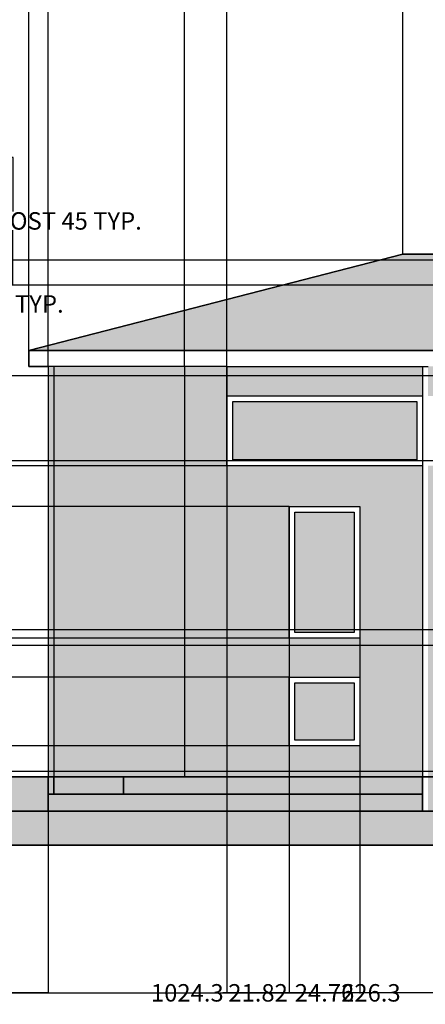
# Model space of a CAD drawing. Units: inches. Extents: x -655 to 499, y 20 to 616.
# Tile 4 of 7: x -137 to 5, y 20 to 365. Entities that reach past the tile are written whole.
import ezdxf

# ---------------------------------------------------------------- set-up
doc = ezdxf.new("R2010")
doc.units = ezdxf.units.IN
doc.header["$MEASUREMENT"] = 0
for name, color, linetype, lineweight in [('A-ANNO-DIMS', 2, 'Continuous', 18), ('A-DOOR', 4, 'Continuous', 25), ('A-ELEV', 7, 'Continuous', 35), ('A-ELEV-PATT', 9, 'Continuous', 13), ('A-ROOF', 1, 'Continuous', 35), ('C-TOPO', 18, 'Continuous', 18)]:
    doc.layers.add(name, color=color, linetype=linetype, lineweight=lineweight)
doc.styles.get("Standard").update_dxf_attribs({"font": 'arial.ttf'})
doc.dimstyles.get("Standard").update_dxf_attribs({"dimtxt": 6.125, "dimasz": 0.18, "dimexe": 0.18, "dimexo": 0.0625, "dimgap": 0.09, "dimtad": 0, "dimtih": 1, "dimtoh": 1, "dimdec": 4, "dimzin": 0, "dimdsep": 46, "dimlunit": 4, "dimtxsty": 'Standard', "dimcen": 0.09, "dimadec": 0, "dimazin": 0, "dimtfac": 1, "dimtdec": 4, "dimtofl": 0, "dimtmove": 0, "dimatfit": 3, "dimfxl": 1, "dimtolj": 1, "dimtzin": 0, "dimarcsym": 0})

# ---------------------------------------------------------------- blocks, each defined once
blk = doc.blocks.new('DOOR-LEAF-PANEL')
for points in [[(0, 122.75), (68.54, 122.75), (68.54, 98.27), (0, 98.27)], [(2, 120.75), (66.54, 120.75), (66.54, 100.27), (2, 100.27)], [(21.82, 83.95), (46.58, 83.95), (46.58, 37.78), (21.82, 37.78)], [(23.82, 81.95), (44.58, 81.95), (44.58, 39.78), (23.82, 39.78)], [(21.82, 24.14), (46.58, 24.14), (46.58, 0), (21.82, 0)], [(23.82, 22.14), (44.58, 22.14), (44.58, 2), (23.82, 2)]]:
    blk.add_lwpolyline(points, close=True)
blk = doc.blocks.new('*D4')
at = {"layer": 'A-ANNO-DIMS', "color": 0, "lineweight": -2, "transparency": 16777216}
for p, q in [((-145.9, 317.05), (-139.06, 317.05)), ((-139.24, 316.87), (-139.24, 297.92)), ((-139.24, 272.44), (-139.24, 291.4)), ((-145.9, 272.26), (-139.06, 272.26))]:
    blk.add_line(p, q, dxfattribs=at)
at = {"layer": 'A-ANNO-DIMS', "color": 0, "transparency": 16777216}
for points in [[(-139.27, 316.87), (-139.21, 316.87), (-139.24, 317.05)], [(-139.27, 272.44), (-139.21, 272.44), (-139.24, 272.26)]]:
    blk.add_solid(points, dxfattribs=at)
at = {"layer": 'Defpoints', "color": 0, "transparency": 16777216}
for p in [(-145.96, 317.05), (-139.24, 317.05), (-145.96, 272.26)]:
    blk.add_point(p, dxfattribs=at)
at = {"layer": 'A-ANNO-DIMS', "color": 0, "transparency": 16777216, "insert": (-139.24, 294.66), "char_height": 6.125, "attachment_point": 5}
blk.add_mtext('\\A1;BALCONY POST 45 TYP.', dxfattribs=at)
blk = doc.blocks.new('*D5')
at = {"layer": 'A-ANNO-DIMS', "color": 0, "lineweight": -2, "transparency": 16777216}
for p, q in [((-150.77, 272.2), (-150.77, 265.36)), ((-145.96, 272.2), (-145.96, 265.36)), ((-150.59, 265.54), (-146.14, 265.54)), ((-145.96, 265.54), (-145.78, 265.54))]:
    blk.add_line(p, q, dxfattribs=at)
at = {"layer": 'A-ANNO-DIMS', "color": 0, "transparency": 16777216}
for points in [[(-150.59, 265.57), (-150.59, 265.51), (-150.77, 265.54)], [(-146.14, 265.57), (-146.14, 265.51), (-145.96, 265.54)]]:
    blk.add_solid(points, dxfattribs=at)
at = {"layer": 'Defpoints', "color": 0, "transparency": 16777216}
for p in [(-150.77, 272.26), (-145.96, 272.26), (-145.96, 265.54)]:
    blk.add_point(p, dxfattribs=at)
at = {"layer": 'A-ANNO-DIMS', "color": 0, "transparency": 16777216, "insert": (-133.16, 265.54), "char_height": 6.125, "attachment_point": 5}
blk.add_mtext('\\A1;5 TYP.', dxfattribs=at)
blk = doc.blocks.new('*D10')
at = {"layer": 'A-ANNO-DIMS', "color": 0, "lineweight": -2, "transparency": 16777216}
for p, q in [((434.11, 393.11), (434.11, 23.7)), ((-590.16, 75.57), (-590.16, 23.7)), ((-589.98, 23.88), (-90.54, 23.88)), ((433.93, 23.88), (-65.51, 23.88))]:
    blk.add_line(p, q, dxfattribs=at)
at = {"layer": 'A-ANNO-DIMS', "color": 0, "transparency": 16777216}
for points in [[(-589.98, 23.91), (-589.98, 23.85), (-590.16, 23.88)], [(433.93, 23.91), (433.93, 23.85), (434.11, 23.88)]]:
    blk.add_solid(points, dxfattribs=at)
at = {"layer": 'Defpoints', "color": 0, "transparency": 16777216}
for p in [(434.11, 393.17), (-590.16, 75.63), (434.11, 23.88)]:
    blk.add_point(p, dxfattribs=at)
at = {"layer": 'A-ANNO-DIMS', "color": 0, "transparency": 16777216, "insert": (-78.02, 23.88), "char_height": 6.125, "attachment_point": 5}
blk.add_mtext('\\A1;1024.3', dxfattribs=at)
blk = doc.blocks.new('*D14')
at = {"layer": 'A-ANNO-DIMS', "color": 0, "lineweight": -2, "transparency": 16777216}
for p, q in [((-229.01, 101.57), (-229.01, 23.7)), ((-126.81, 99.57), (-126.81, 23.7)), ((-228.83, 23.88), (-188.01, 23.88)), ((-126.99, 23.88), (-167.8, 23.88))]:
    blk.add_line(p, q, dxfattribs=at)
at = {"layer": 'A-ANNO-DIMS', "color": 0, "transparency": 16777216}
for points in [[(-228.83, 23.91), (-228.83, 23.85), (-229.01, 23.88)], [(-126.99, 23.91), (-126.99, 23.85), (-126.81, 23.88)]]:
    blk.add_solid(points, dxfattribs=at)
at = {"layer": 'Defpoints', "color": 0, "transparency": 16777216}
for p in [(-229.01, 101.63), (-126.81, 99.63), (-126.81, 23.88)]:
    blk.add_point(p, dxfattribs=at)
at = {"layer": 'A-ANNO-DIMS', "color": 0, "transparency": 16777216, "insert": (-177.91, 23.88), "char_height": 6.125, "attachment_point": 5}
blk.add_mtext('\\A1;102.2', dxfattribs=at)
blk = doc.blocks.new('*D15')
at = {"layer": 'A-ANNO-DIMS', "color": 0, "lineweight": -2, "transparency": 16777216}
for p, q in [((-126.81, 99.57), (-126.81, 23.7)), ((99.5, 93.57), (99.5, 23.7)), ((-126.63, 23.88), (-24.13, 23.88)), ((99.32, 23.88), (-3.18, 23.88))]:
    blk.add_line(p, q, dxfattribs=at)
at = {"layer": 'A-ANNO-DIMS', "color": 0, "transparency": 16777216}
for points in [[(-126.63, 23.91), (-126.63, 23.85), (-126.81, 23.88)], [(99.32, 23.91), (99.32, 23.85), (99.5, 23.88)]]:
    blk.add_solid(points, dxfattribs=at)
at = {"layer": 'Defpoints', "color": 0, "transparency": 16777216}
for p in [(-126.81, 99.63), (99.5, 93.63), (99.5, 23.88)]:
    blk.add_point(p, dxfattribs=at)
at = {"layer": 'A-ANNO-DIMS', "color": 0, "transparency": 16777216, "insert": (-13.65, 23.88), "char_height": 6.125, "attachment_point": 5}
blk.add_mtext('\\A1;226.3', dxfattribs=at)
blk = doc.blocks.new('*D21')
at = {"layer": 'A-ANNO-DIMS', "color": 0, "lineweight": -2, "transparency": 16777216}
for p, q in [((179.11, 559.78), (486.04, 559.78)), ((485.86, 559.6), (485.86, 320.92)), ((485.86, 75.81), (485.86, 314.49)), ((-590.1, 75.63), (486.04, 75.63))]:
    blk.add_line(p, q, dxfattribs=at)
at = {"layer": 'A-ANNO-DIMS', "color": 0, "transparency": 16777216}
for points in [[(485.83, 559.6), (485.89, 559.6), (485.86, 559.78)], [(485.83, 75.81), (485.89, 75.81), (485.86, 75.63)]]:
    blk.add_solid(points, dxfattribs=at)
at = {"layer": 'Defpoints', "color": 0, "transparency": 16777216}
for p in [(179.05, 559.78), (485.86, 559.78), (-590.16, 75.63)]:
    blk.add_point(p, dxfattribs=at)
at = {"layer": 'A-ANNO-DIMS', "color": 0, "transparency": 16777216, "insert": (485.86, 317.7), "char_height": 6.125, "attachment_point": 5}
blk.add_mtext('\\A1;484.15', dxfattribs=at)
blk = doc.blocks.new('*D35')
at = {"layer": 'A-ANNO-DIMS', "color": 0, "lineweight": -2, "transparency": 16777216}
for p, q in [((-244.62, 280.97), (486.04, 280.97)), ((485.86, 280.79), (485.86, 279.83)), ((485.86, 272.44), (485.86, 273.4)), ((-226.95, 272.26), (486.04, 272.26))]:
    blk.add_line(p, q, dxfattribs=at)
at = {"layer": 'A-ANNO-DIMS', "color": 0, "transparency": 16777216}
for points in [[(485.83, 280.79), (485.89, 280.79), (485.86, 280.97)], [(485.83, 272.44), (485.89, 272.44), (485.86, 272.26)]]:
    blk.add_solid(points, dxfattribs=at)
at = {"layer": 'Defpoints', "color": 0, "transparency": 16777216}
for p in [(-244.69, 280.97), (-227.01, 272.26), (485.86, 272.26)]:
    blk.add_point(p, dxfattribs=at)
at = {"layer": 'A-ANNO-DIMS', "color": 0, "transparency": 16777216, "insert": (485.86, 276.61), "char_height": 6.125, "attachment_point": 5}
blk.add_mtext('\\A1;8.706', dxfattribs=at)
blk = doc.blocks.new('*D48')
at = {"layer": 'A-ANNO-DIMS', "color": 0, "lineweight": -2, "transparency": 16777216}
for p, q in [((-228.95, 145.8), (486.04, 145.8)), ((485.86, 145.62), (485.86, 126.88)), ((485.86, 101.81), (485.86, 120.55)), ((-228.95, 101.63), (486.04, 101.63))]:
    blk.add_line(p, q, dxfattribs=at)
at = {"layer": 'A-ANNO-DIMS', "color": 0, "transparency": 16777216}
for points in [[(485.83, 145.62), (485.89, 145.62), (485.86, 145.8)], [(485.83, 101.81), (485.89, 101.81), (485.86, 101.63)]]:
    blk.add_solid(points, dxfattribs=at)
at = {"layer": 'Defpoints', "color": 0, "transparency": 16777216}
for p in [(-229.01, 145.8), (485.86, 145.8), (-229.01, 101.63)]:
    blk.add_point(p, dxfattribs=at)
at = {"layer": 'A-ANNO-DIMS', "color": 0, "transparency": 16777216, "insert": (485.86, 123.72), "char_height": 6.125, "attachment_point": 5}
blk.add_mtext('\\A1;44.17', dxfattribs=at)
blk = doc.blocks.new('*D49')
at = {"layer": 'A-ANNO-DIMS', "color": 0, "lineweight": -2, "transparency": 16777216}
for p, q in [((-229.3, 210.64), (486.04, 210.64)), ((485.86, 210.46), (485.86, 184.21)), ((485.86, 151.52), (485.86, 177.77)), ((-229.3, 151.34), (486.04, 151.34))]:
    blk.add_line(p, q, dxfattribs=at)
at = {"layer": 'A-ANNO-DIMS', "color": 0, "transparency": 16777216}
for points in [[(485.83, 210.46), (485.89, 210.46), (485.86, 210.64)], [(485.83, 151.52), (485.89, 151.52), (485.86, 151.34)]]:
    blk.add_solid(points, dxfattribs=at)
at = {"layer": 'Defpoints', "color": 0, "transparency": 16777216}
for p in [(-229.36, 210.64), (485.86, 210.64), (-229.36, 151.34)]:
    blk.add_point(p, dxfattribs=at)
at = {"layer": 'A-ANNO-DIMS', "color": 0, "transparency": 16777216, "insert": (485.86, 180.99), "char_height": 6.125, "attachment_point": 5}
blk.add_mtext('\\A1;59.3', dxfattribs=at)
blk = doc.blocks.new('*D51')
at = {"layer": 'A-ANNO-DIMS', "color": 0, "lineweight": -2, "transparency": 16777216}
for p, q in [((-228.95, 240.42), (486.04, 240.42)), ((485.86, 240.24), (485.86, 228.75)), ((485.86, 210.82), (485.86, 222.31)), ((-228.88, 210.64), (486.04, 210.64))]:
    blk.add_line(p, q, dxfattribs=at)
at = {"layer": 'A-ANNO-DIMS', "color": 0, "transparency": 16777216}
for points in [[(485.83, 240.24), (485.89, 240.24), (485.86, 240.42)], [(485.83, 210.82), (485.89, 210.82), (485.86, 210.64)]]:
    blk.add_solid(points, dxfattribs=at)
at = {"layer": 'Defpoints', "color": 0, "transparency": 16777216}
for p in [(-229.01, 240.42), (485.86, 240.42), (-228.94, 210.64)]:
    blk.add_point(p, dxfattribs=at)
at = {"layer": 'A-ANNO-DIMS', "color": 0, "transparency": 16777216, "insert": (485.86, 225.53), "char_height": 6.125, "attachment_point": 5}
blk.add_mtext('\\A1;29.776', dxfattribs=at)
blk = doc.blocks.new('*D55')
at = {"layer": 'A-ANNO-DIMS', "color": 0, "lineweight": -2, "transparency": 16777216}
for p, q in [((-133.53, 249.26), (-133.53, 611.71)), ((-133.35, 611.53), (-80.53, 611.53)), ((-2.68, 611.53), (-55.5, 611.53)), ((-2.5, 283.02), (-2.5, 611.71))]:
    blk.add_line(p, q, dxfattribs=at)
at = {"layer": 'A-ANNO-DIMS', "color": 0, "transparency": 16777216}
for points in [[(-133.35, 611.56), (-133.35, 611.5), (-133.53, 611.53)], [(-2.68, 611.56), (-2.68, 611.5), (-2.5, 611.53)]]:
    blk.add_solid(points, dxfattribs=at)
at = {"layer": 'Defpoints', "color": 0, "transparency": 16777216}
for p in [(-2.5, 611.53), (-2.5, 282.96), (-133.53, 249.2)]:
    blk.add_point(p, dxfattribs=at)
at = {"layer": 'A-ANNO-DIMS', "color": 0, "transparency": 16777216, "insert": (-68.01, 611.53), "char_height": 6.125, "attachment_point": 5}
blk.add_mtext('\\A1;131.03', dxfattribs=at)
blk = doc.blocks.new('*D56')
at = {"layer": 'A-ANNO-DIMS', "color": 0, "lineweight": -2, "transparency": 16777216}
for p, q in [((-2.5, 283.02), (-2.5, 611.71)), ((-2.32, 611.53), (46.26, 611.53)), ((115.13, 611.53), (66.55, 611.53)), ((115.31, 249.31), (115.31, 611.71))]:
    blk.add_line(p, q, dxfattribs=at)
at = {"layer": 'A-ANNO-DIMS', "color": 0, "transparency": 16777216}
for points in [[(-2.32, 611.56), (-2.32, 611.5), (-2.5, 611.53)], [(115.13, 611.56), (115.13, 611.5), (115.31, 611.53)]]:
    blk.add_solid(points, dxfattribs=at)
at = {"layer": 'Defpoints', "color": 0, "transparency": 16777216}
for p in [(115.31, 611.53), (-2.5, 282.96), (115.31, 249.25)]:
    blk.add_point(p, dxfattribs=at)
at = {"layer": 'A-ANNO-DIMS', "color": 0, "transparency": 16777216, "insert": (56.41, 611.53), "char_height": 6.125, "attachment_point": 5}
blk.add_mtext('\\A1;117.8', dxfattribs=at)
blk = doc.blocks.new('*D59')
at = {"layer": 'A-ANNO-DIMS', "color": 0, "lineweight": -2, "transparency": 16777216}
for p, q in [((-126.81, 243.69), (-126.81, 611.71)), ((-126.63, 611.53), (-113.42, 611.53)), ((-79.15, 611.53), (-92.35, 611.53)), ((-78.97, 243.69), (-78.97, 611.71))]:
    blk.add_line(p, q, dxfattribs=at)
at = {"layer": 'A-ANNO-DIMS', "color": 0, "transparency": 16777216}
for points in [[(-126.63, 611.56), (-126.63, 611.5), (-126.81, 611.53)], [(-79.15, 611.56), (-79.15, 611.5), (-78.97, 611.53)]]:
    blk.add_solid(points, dxfattribs=at)
at = {"layer": 'Defpoints', "color": 0, "transparency": 16777216}
for p in [(-78.97, 611.53), (-126.81, 243.63), (-78.97, 243.63)]:
    blk.add_point(p, dxfattribs=at)
at = {"layer": 'A-ANNO-DIMS', "color": 0, "transparency": 16777216, "insert": (-102.89, 611.53), "char_height": 6.125, "attachment_point": 5}
blk.add_mtext('\\A1;47.84', dxfattribs=at)
blk = doc.blocks.new('*D60')
at = {"layer": 'A-ANNO-DIMS', "color": 0, "lineweight": -2, "transparency": 16777216}
for p, q in [((-78.97, 243.69), (-78.97, 611.71)), ((-78.79, 611.53), (-64.3, 611.53)), ((-64.12, 233.34), (-64.12, 611.71)), ((-64.12, 611.53), (-63.94, 611.53))]:
    blk.add_line(p, q, dxfattribs=at)
at = {"layer": 'A-ANNO-DIMS', "color": 0, "transparency": 16777216}
for points in [[(-78.79, 611.56), (-78.79, 611.5), (-78.97, 611.53)], [(-64.3, 611.56), (-64.3, 611.5), (-64.12, 611.53)]]:
    blk.add_solid(points, dxfattribs=at)
at = {"layer": 'Defpoints', "color": 0, "transparency": 16777216}
for p in [(-64.12, 611.53), (-78.97, 243.63), (-64.12, 233.27)]:
    blk.add_point(p, dxfattribs=at)
at = {"layer": 'A-ANNO-DIMS', "color": 0, "transparency": 16777216, "insert": (-53.78, 611.53), "char_height": 6.125, "attachment_point": 5}
blk.add_mtext('\\A1;14.85', dxfattribs=at)
blk = doc.blocks.new('*D61')
at = {"layer": 'A-ANNO-DIMS', "color": 0, "lineweight": -2, "transparency": 16777216}
for p, q in [((-64.12, 233.34), (-64.12, 611.71)), ((-63.94, 611.53), (0.16, 611.53)), ((89.22, 611.53), (25.13, 611.53)), ((89.4, 243.69), (89.4, 611.71))]:
    blk.add_line(p, q, dxfattribs=at)
at = {"layer": 'A-ANNO-DIMS', "color": 0, "transparency": 16777216}
for points in [[(-63.94, 611.56), (-63.94, 611.5), (-64.12, 611.53)], [(89.22, 611.56), (89.22, 611.5), (89.4, 611.53)]]:
    blk.add_solid(points, dxfattribs=at)
at = {"layer": 'Defpoints', "color": 0, "transparency": 16777216}
for p in [(89.4, 611.53), (89.4, 243.63), (-64.12, 233.27)]:
    blk.add_point(p, dxfattribs=at)
at = {"layer": 'A-ANNO-DIMS', "color": 0, "transparency": 16777216, "insert": (12.64, 611.53), "char_height": 6.125, "attachment_point": 5}
blk.add_mtext('\\A1;153.52', dxfattribs=at)
blk = doc.blocks.new('*D65')
at = {"layer": 'A-ANNO-DIMS', "color": 0, "lineweight": -2, "transparency": 16777216}
for p, q in [((-64.12, 208.73), (-64.12, 23.7)), ((-42.3, 194.41), (-42.3, 23.7)), ((-63.94, 23.88), (-63.65, 23.88)), ((-42.48, 23.88), (-42.76, 23.88))]:
    blk.add_line(p, q, dxfattribs=at)
at = {"layer": 'A-ANNO-DIMS', "color": 0, "transparency": 16777216}
for points in [[(-63.94, 23.91), (-63.94, 23.85), (-64.12, 23.88)], [(-42.48, 23.91), (-42.48, 23.85), (-42.3, 23.88)]]:
    blk.add_solid(points, dxfattribs=at)
at = {"layer": 'Defpoints', "color": 0, "transparency": 16777216}
for p in [(-64.12, 208.79), (-42.3, 194.47), (-42.3, 23.88)]:
    blk.add_point(p, dxfattribs=at)
at = {"layer": 'A-ANNO-DIMS', "color": 0, "transparency": 16777216, "insert": (-53.21, 23.88), "char_height": 6.125, "attachment_point": 5}
blk.add_mtext('\\A1;21.82', dxfattribs=at)
blk = doc.blocks.new('*D66')
at = {"layer": 'A-ANNO-DIMS', "color": 0, "lineweight": -2, "transparency": 16777216}
for p, q in [((-42.3, 194.41), (-42.3, 23.7)), ((-17.54, 194.41), (-17.54, 23.7)), ((-42.12, 23.88), (-40.39, 23.88)), ((-17.72, 23.88), (-19.44, 23.88))]:
    blk.add_line(p, q, dxfattribs=at)
at = {"layer": 'A-ANNO-DIMS', "color": 0, "transparency": 16777216}
for points in [[(-42.12, 23.91), (-42.12, 23.85), (-42.3, 23.88)], [(-17.72, 23.91), (-17.72, 23.85), (-17.54, 23.88)]]:
    blk.add_solid(points, dxfattribs=at)
at = {"layer": 'Defpoints', "color": 0, "transparency": 16777216}
for p in [(-42.3, 194.47), (-17.54, 194.47), (-17.54, 23.88)]:
    blk.add_point(p, dxfattribs=at)
at = {"layer": 'A-ANNO-DIMS', "color": 0, "transparency": 16777216, "insert": (-29.92, 23.88), "char_height": 6.125, "attachment_point": 5}
blk.add_mtext('\\A1;24.76', dxfattribs=at)
blk = doc.blocks.new('*D67')
at = {"layer": 'A-ANNO-DIMS', "color": 0, "lineweight": -2, "transparency": 16777216}
for p, q in [((-42.36, 110.53), (-642.09, 110.53)), ((-641.91, 110.35), (-641.91, 108.29)), ((-641.91, 99.81), (-641.91, 101.86)), ((-64.18, 99.63), (-642.09, 99.63))]:
    blk.add_line(p, q, dxfattribs=at)
at = {"layer": 'A-ANNO-DIMS', "color": 0, "transparency": 16777216}
for points in [[(-641.94, 110.35), (-641.88, 110.35), (-641.91, 110.53)], [(-641.94, 99.81), (-641.88, 99.81), (-641.91, 99.63)]]:
    blk.add_solid(points, dxfattribs=at)
at = {"layer": 'Defpoints', "color": 0, "transparency": 16777216}
for p in [(-42.3, 110.53), (-641.91, 99.63), (-64.12, 99.63)]:
    blk.add_point(p, dxfattribs=at)
at = {"layer": 'A-ANNO-DIMS', "color": 0, "transparency": 16777216, "insert": (-641.91, 105.08), "char_height": 6.125, "attachment_point": 5}
blk.add_mtext('\\A1;10.896', dxfattribs=at)
blk = doc.blocks.new('*D68')
at = {"layer": 'A-ANNO-DIMS', "color": 0, "lineweight": -2, "transparency": 16777216}
for p, q in [((-42.36, 134.67), (-642.09, 134.67)), ((-641.91, 134.49), (-641.91, 125.76)), ((-641.91, 110.71), (-641.91, 119.43)), ((-42.36, 110.53), (-642.09, 110.53))]:
    blk.add_line(p, q, dxfattribs=at)
at = {"layer": 'A-ANNO-DIMS', "color": 0, "transparency": 16777216}
for points in [[(-641.94, 134.49), (-641.88, 134.49), (-641.91, 134.67)], [(-641.94, 110.71), (-641.88, 110.71), (-641.91, 110.53)]]:
    blk.add_solid(points, dxfattribs=at)
at = {"layer": 'Defpoints', "color": 0, "transparency": 16777216}
for p in [(-641.91, 134.67), (-42.3, 134.67), (-42.3, 110.53)]:
    blk.add_point(p, dxfattribs=at)
at = {"layer": 'A-ANNO-DIMS', "color": 0, "transparency": 16777216, "insert": (-641.91, 122.6), "char_height": 6.125, "attachment_point": 5}
blk.add_mtext('\\A1;24.14', dxfattribs=at)
blk = doc.blocks.new('*D69')
at = {"layer": 'A-ANNO-DIMS', "color": 0, "lineweight": -2, "transparency": 16777216}
for p, q in [((-42.36, 148.31), (-642.09, 148.31)), ((-641.91, 148.13), (-641.91, 144.71)), ((-641.91, 134.85), (-641.91, 138.27)), ((-42.36, 134.67), (-642.09, 134.67))]:
    blk.add_line(p, q, dxfattribs=at)
at = {"layer": 'A-ANNO-DIMS', "color": 0, "transparency": 16777216}
for points in [[(-641.94, 148.13), (-641.88, 148.13), (-641.91, 148.31)], [(-641.94, 134.85), (-641.88, 134.85), (-641.91, 134.67)]]:
    blk.add_solid(points, dxfattribs=at)
at = {"layer": 'Defpoints', "color": 0, "transparency": 16777216}
for p in [(-641.91, 148.31), (-42.3, 148.31), (-42.3, 134.67)]:
    blk.add_point(p, dxfattribs=at)
at = {"layer": 'A-ANNO-DIMS', "color": 0, "transparency": 16777216, "insert": (-641.91, 141.49), "char_height": 6.125, "attachment_point": 5}
blk.add_mtext('\\A1;13.64', dxfattribs=at)
blk = doc.blocks.new('*D70')
at = {"layer": 'A-ANNO-DIMS', "color": 0, "lineweight": -2, "transparency": 16777216}
for p, q in [((-42.36, 194.47), (-642.09, 194.47)), ((-641.91, 194.29), (-641.91, 174.61)), ((-641.91, 148.49), (-641.91, 168.17)), ((-42.36, 148.31), (-642.09, 148.31))]:
    blk.add_line(p, q, dxfattribs=at)
at = {"layer": 'A-ANNO-DIMS', "color": 0, "transparency": 16777216}
for points in [[(-641.94, 194.29), (-641.88, 194.29), (-641.91, 194.47)], [(-641.94, 148.49), (-641.88, 148.49), (-641.91, 148.31)]]:
    blk.add_solid(points, dxfattribs=at)
at = {"layer": 'Defpoints', "color": 0, "transparency": 16777216}
for p in [(-641.91, 194.47), (-42.3, 194.47), (-42.3, 148.31)]:
    blk.add_point(p, dxfattribs=at)
at = {"layer": 'A-ANNO-DIMS', "color": 0, "transparency": 16777216, "insert": (-641.91, 171.39), "char_height": 6.125, "attachment_point": 5}
blk.add_mtext('\\A1;46.16', dxfattribs=at)
blk = doc.blocks.new('*D71')
at = {"layer": 'A-ANNO-DIMS', "color": 0, "lineweight": -2, "transparency": 16777216}
for p, q in [((-64.18, 208.79), (-642.09, 208.79)), ((-641.91, 208.61), (-641.91, 204.85)), ((-641.91, 194.65), (-641.91, 198.41)), ((-42.36, 194.47), (-642.09, 194.47))]:
    blk.add_line(p, q, dxfattribs=at)
at = {"layer": 'A-ANNO-DIMS', "color": 0, "transparency": 16777216}
for points in [[(-641.94, 208.61), (-641.88, 208.61), (-641.91, 208.79)], [(-641.94, 194.65), (-641.88, 194.65), (-641.91, 194.47)]]:
    blk.add_solid(points, dxfattribs=at)
at = {"layer": 'Defpoints', "color": 0, "transparency": 16777216}
for p in [(-641.91, 208.79), (-64.12, 208.79), (-42.3, 194.47)]:
    blk.add_point(p, dxfattribs=at)
at = {"layer": 'A-ANNO-DIMS', "color": 0, "transparency": 16777216, "insert": (-641.91, 201.63), "char_height": 6.125, "attachment_point": 5}
blk.add_mtext('\\A1;14.32', dxfattribs=at)

msp = doc.modelspace()

# ---------------------------------------------------------------- hatches: boundary and pattern name
at = {"layer": 'A-ELEV-PATT'}
h = msp.add_hatch(color=256, dxfattribs=at)
h.dxf.hatch_style = 1
h.paths.add_polyline_path([(-140.0489, 272.2618), (-399.3758, 272.2618), (-399.3758, 249.8418), (-399.3758, 248.5179), (-366.9446, 248.7444), (-209.8047, 249.8418), (-183.5755, 249.8418), (-140.0489, 249.8418)])
h.paths.add_polyline_path([(-211.7589, 317.0515), (-216.5713, 317.0515), (-216.5713, 272.2618), (-211.7589, 272.2618)])
h.paths.add_polyline_path([(-145.96, 317.0515), (-150.7725, 317.0515), (-150.7725, 272.2618), (-145.96, 272.2618)])
h.paths.add_polyline_path([(-140.5198, 321.4867), (-402.0739, 321.4867), (-402.0739, 317.0515), (-390.1757, 317.0515), (-385.3633, 317.0515), (-150.7725, 317.0515), (-145.96, 317.0515), (-140.5198, 317.0515)])
h.paths.add_polyline_path([(-269.7123, 317.0515), (-274.5248, 317.0515), (-274.5248, 272.2618), (-269.7123, 272.2618)])
h.paths.add_polyline_path([(-329.7837, 317.0515), (-334.5961, 317.0515), (-334.5961, 280.9678), (-329.7837, 280.9678)])
h.paths.add_polyline_path([(-329.7837, 280.9678), (-334.5961, 280.9678), (-334.5961, 272.2618), (-329.7837, 272.2618)])
h.paths.add_polyline_path([(-385.3633, 317.0515), (-390.1757, 317.0515), (-390.1757, 272.2618), (-385.3633, 272.2618)])
h.paths.add_polyline_path([(-229.0087, 240.4184), (-354.3532, 240.4184), (-354.2854, 210.6425), (-315.9956, 210.6425), (-315.9956, 210.9348), (-277.6793, 210.7995), (-277.6793, 210.6425), (-273.1052, 210.6425), (-273.1052, 210.7995), (-229.3637, 210.6425), (-229.0087, 210.6425)])
h.paths.add_polyline_path([(-229.0087, 145.8007), (-354.3532, 145.8007), (-354.3532, 101.6296), (-229.0087, 101.6296)])
h.paths.add_polyline_path([(-229.0087, 210.6425), (-229.3637, 210.6425), (-229.3637, 151.3385), (-273.1052, 151.4955), (-273.1052, 210.6425), (-277.6793, 210.6425), (-277.6793, 151.4955), (-315.9956, 151.6308), (-315.9956, 210.6425), (-318.9742, 210.6425), (-318.9742, 151.3385), (-354.3532, 151.3385), (-354.3532, 145.8007), (-229.0087, 145.8007)])
h.paths.add_polyline_path([(-229.0087, 247.8418), (-354.3532, 247.8418), (-354.3532, 240.4184), (-229.0087, 240.4184)])
h.paths.add_polyline_path([(4.4271, 93.6296), (-100.4134, 93.6296), (-124.8077, 93.6296), (-126.8077, 93.6296), (-126.8077, 87.6296), (4.4271, 87.6296)])
h.paths.add_polyline_path([(4.4271, 99.6296), (-100.4134, 99.6296), (-100.4134, 93.6296), (4.4271, 93.6296)])
h.paths.add_polyline_path([(99.4982, 99.6296), (6.4271, 99.6296), (6.4271, 93.6296), (99.4982, 93.6296)])
h.paths.add_polyline_path([(99.4982, 93.6296), (6.4271, 93.6296), (6.4271, 87.6296), (99.4982, 87.6296)])
h.paths.add_polyline_path([(304.2843, 311.436), (230.0144, 311.076), (230.0144, 282.9577), (270.6361, 282.9577), (304.4665, 273.8535)])
h.paths.add_polyline_path([(304.1054, 348.3371), (304.1054, 356.2861), (230.0144, 356.2861), (230.0144, 348.3443), (230.0144, 311.076), (304.2843, 311.436)])
h.paths.add_polyline_path([(255.5586, 316.5111), (255.5586, 350.0185), (275.6848, 350.0185), (275.6848, 316.5111)], flags=16)
h.paths.add_polyline_path([(278.0676, 316.5111), (278.0676, 350.0185), (301.4074, 350.0185), (301.4074, 316.5111)], flags=16)
h.paths.add_polyline_path([(253.2029, 316.5111), (233.8107, 316.5111), (233.8107, 350.0185), (253.2029, 350.0185)], flags=16)
h.paths.add_polyline_path([(179.0482, 559.7795), (153.2347, 535.8185), (165.0976, 535.8185), (192.9989, 535.8185), (201.2897, 535.8185)])
h.paths.add_polyline_path([(347.8163, 516.7932), (322.0028, 492.8322), (333.8657, 492.8322), (361.7669, 492.8322), (370.0577, 492.8322)])
h = msp.add_hatch(color=256, dxfattribs=at)
h.dxf.hatch_style = 1
h.paths.add_polyline_path([(-329.7837, 350.1333), (-347.0336, 350.1333), (-347.0336, 321.4867), (-329.7837, 321.4867)])
h.paths.add_polyline_path([(-294.1413, 350.1333), (-311.3912, 350.1333), (-311.3912, 321.4867), (-294.1413, 321.4867)])
h.paths.add_polyline_path([(-294.1413, 317.0515), (-311.3912, 317.0515), (-311.3912, 280.9678), (-294.1413, 280.9678)])
h.paths.add_polyline_path([(-334.5961, 317.0515), (-347.0336, 317.0515), (-347.0336, 280.9678), (-334.5961, 280.9678)])
h.paths.add_polyline_path([(-244.6859, 336.719), (-258.4486, 336.719), (-258.4486, 347.0139), (-244.6859, 347.0139), (-244.6859, 350.1333), (-261.9358, 350.1333), (-261.9358, 321.4867), (-244.6859, 321.4867)])
h.paths.add_polyline_path([(-244.6859, 317.0515), (-261.9358, 317.0515), (-261.9358, 280.9678), (-244.6859, 280.9678)])
h.paths.add_polyline_path([(-244.6859, 347.0139), (-258.4486, 347.0139), (-258.4486, 336.719), (-244.6859, 336.719)], flags=17)
h.paths.add_polyline_path([(-318.9742, 210.6425), (-354.3532, 210.6425), (-354.3532, 151.3385), (-318.9742, 151.3385)])
h.paths.add_polyline_path([(-277.6793, 210.6425), (-315.9956, 210.6425), (-315.9956, 151.6308), (-277.6793, 151.4955)])
h.paths.add_polyline_path([(-229.3637, 210.6425), (-273.1052, 210.6425), (-273.1052, 151.4955), (-229.3637, 151.3385)])
h.paths.add_polyline_path([(-19.537, 192.4712), (-40.2951, 192.4712), (-40.2951, 150.3082), (-19.537, 150.3082)])
h.paths.add_polyline_path([(2.4271, 231.274), (-62.1158, 231.274), (-62.1158, 210.7923), (2.4271, 210.7923)])
h.paths.add_polyline_path([(72.97, 231.274), (8.4271, 231.274), (8.4271, 210.7923), (72.97, 210.7923)])
h.paths.add_polyline_path([(51.0059, 192.4712), (30.2478, 192.4712), (30.2478, 150.3082), (51.0059, 150.3082)])
h.paths.add_polyline_path([(51.0059, 132.6671), (30.2478, 132.6671), (30.2478, 112.5254), (51.0059, 112.5254)])
h.paths.add_polyline_path([(-19.537, 132.6671), (-40.2951, 132.6671), (-40.2951, 112.5254), (-19.537, 112.5254)])
h.paths.add_polyline_path([(275.6848, 350.0185), (255.5586, 350.0185), (255.5586, 316.5111), (275.6848, 316.5111)])
h.paths.add_polyline_path([(301.4074, 350.0185), (278.0676, 350.0185), (278.0676, 316.5111), (301.4074, 316.5111)])
h.paths.add_polyline_path([(253.2029, 350.0185), (233.8107, 350.0185), (233.8107, 316.5111), (253.2029, 316.5111)])
h = msp.add_hatch(color=256, dxfattribs=at)
h.dxf.hatch_style = 1
h.paths.add_polyline_path([(-126.8077, 93.6296), (-126.8077, 99.6296), (-145.6102, 99.6296), (-209.8047, 99.6296), (-366.9446, 98.5321), (-366.9446, 99.6296), (-506.835, 99.6296), (-573.6788, 99.6296), (-573.6788, 87.6296), (-506.835, 87.6296), (-161.7817, 87.6296), (-126.8077, 87.6296)])
h.paths.add_polyline_path([(419.8436, 99.6296), (99.4982, 99.6296), (99.4982, 87.6296), (419.8436, 87.6296)])
h.paths.add_polyline_path([(-100.4134, 99.6296), (-124.8077, 99.6296), (-124.8077, 93.6296), (-100.4134, 93.6296)])
h.paths.add_polyline_path([(-124.8077, 243.6296), (-126.8077, 243.6296), (-126.8077, 99.6296), (-124.8077, 99.6296)])
h.paths.add_polyline_path([(-124.8077, 99.6296), (-126.8077, 99.6296), (-126.8077, 93.6296), (-124.8077, 93.6296)])
h = msp.add_hatch(color=256, dxfattribs=at)
h.dxf.hatch_style = 1
h.paths.add_polyline_path([(-78.9669, 243.6296), (-124.8077, 243.6296), (-124.8077, 99.6296), (-78.9669, 99.6296)])
h.paths.add_polyline_path([(109.2763, 243.6296), (100.3937, 243.6296), (89.4008, 243.6296), (89.4008, 99.6296), (99.4982, 99.6296), (109.2763, 99.6296)])
h = msp.add_hatch(color=256, dxfattribs=at)
h.dxf.hatch_style = 1
h.paths.add_polyline_path([(-64.1158, 243.6296), (-78.9669, 243.6296), (-78.9669, 99.6296), (-64.1158, 99.6296)])
h.paths.add_polyline_path([(74.97, 243.6296), (18.4987, 243.6296), (6.4271, 243.6296), (6.4271, 233.274), (74.97, 233.274)])
h.paths.add_polyline_path([(4.4271, 243.6296), (4.3518, 243.6296), (4.0451, 243.6296), (-52.0442, 243.6296), (-64.1158, 243.6296), (-64.1158, 233.274), (4.4271, 233.274)])
h.paths.add_polyline_path([(89.4008, 243.6296), (74.97, 243.6296), (74.97, 233.274), (74.97, 99.6296), (89.4008, 99.6296)])
h.paths.add_polyline_path([(74.97, 208.7923), (6.4271, 208.7923), (6.4271, 99.6296), (74.97, 99.6296)])
h.paths.add_polyline_path([(53.0059, 148.3082), (28.2478, 148.3082), (28.2478, 194.4712), (53.0059, 194.4712)], flags=16)
h.paths.add_polyline_path([(51.0059, 150.3082), (30.2478, 150.3082), (30.2478, 192.4712), (51.0059, 192.4712)], flags=0)
h.paths.add_polyline_path([(53.0059, 134.6671), (53.0059, 110.5254), (28.2478, 110.5254), (28.2478, 134.6671)], flags=16)
h.paths.add_polyline_path([(51.0059, 132.6671), (51.0059, 112.5254), (30.2478, 112.5254), (30.2478, 132.6671)], flags=0)
h.paths.add_polyline_path([(4.4271, 208.7923), (-64.1158, 208.7923), (-64.1158, 99.6296), (4.4271, 99.6296)])
h.paths.add_polyline_path([(-17.537, 148.3082), (-42.2951, 148.3082), (-42.2951, 194.4712), (-17.537, 194.4712)], flags=16)
h.paths.add_polyline_path([(-19.537, 150.3082), (-40.2951, 150.3082), (-40.2951, 192.4712), (-19.537, 192.4712)], flags=0)
h.paths.add_polyline_path([(-17.537, 134.6671), (-17.537, 110.5254), (-42.2951, 110.5254), (-42.2951, 134.6671)], flags=16)
h.paths.add_polyline_path([(-19.537, 132.6671), (-19.537, 112.5254), (-40.2951, 112.5254), (-40.2951, 132.6671)], flags=0)
at = {"layer": 'A-ROOF'}
h = msp.add_hatch(dxfattribs=at)
h.set_pattern_fill('AR-RSHKE', color=256)
h.paths.add_polyline_path([(-5.7434, 500.5192), (-493.0344, 393.1054), (-371.042, 393.1054), (119.6374, 393.1054), (415.7378, 393.1651)])
h.paths.add_polyline_path([(119.638, 282.9577), (-2.4978, 282.9577), (-133.531, 249.2017), (115.3098, 249.2518), (119.638, 250.1911)])
h.paths.add_polyline_path([(270.6361, 282.9577), (119.638, 282.9577), (119.638, 250.1911)], flags=17)
h.paths.add_polyline_path([(270.6361, 282.9577), (119.638, 250.1911), (119.638, 249.2527), (395.6741, 249.3083)])
h.paths.add_polyline_path([(-493.0344, 269.4313), (-534.9108, 229.7008), (-493.0344, 229.7008)])
at = {"layer": 'C-TOPO'}
h = msp.add_hatch(dxfattribs=at)
h.set_pattern_fill('GRAVEL', color=256, scale=2.2)
h.set_pattern_definition([(228.012788, (1.584, 2.2), (-17.6, -19.8), [0.295979, -29.301994]), (184.96974, (1.386, 1.98), (26.4, 2.2), [0.5079096, -50.2830345]), (132.510447, (0.88, 1.936), (22, -24.2), [0.3581336, -35.455272]), (267.27369, (0.022, 1.386), (2.2, 44), [0.4625236, -45.789828]), (292.833654, (0, 0.924), (-11, 26.4), [0.453541, -44.900621]), (357.27369, (0.176, 0.506), (-44, 2.2), [0.4625236, -45.789828]), (37.69424, (0.638, 0.484), (-28.6, -22), [0.611664, -60.554667]), (72.255328, (1.122, 0.858), (15.4, 48.4), [0.5774736, -57.169907]), (121.429566, (1.298, 1.408), (-17.6, 28.6), [0.46409, -45.944961]), (175.23636, (1.056, 1.804), (24.2, -2.2), [0.5298304, -25.961678]), (222.397438, (0.528, 1.848), (-26.4, -24.2), [0.6851856, -67.833425]), (138.814075, (2.2, 1.364), (-15.4, 13.2), [0.233862, -23.1524586]), (171.469234, (2.024, 1.518), (28.6, -4.4), [0.4449214, -44.047325]), (225, (1.584, 1.584), (-2e-16, -2.2), [0.311126, -2.800144]), (203.19859, (1.43, 1.848), (11, 4.4), [0.1675476, -16.587153]), (291.80141, (1.276, 1.782), (-2.2, 6.6), [0.2369466, -11.610416]), (30.96376, (1.364, 1.562), (6.6, 4.4), [0.384844, -12.44325]), (161.56505, (1.694, 1.76), (4.4, -2.2), [0.27828, -6.678731]), (16.38954, (0, 1.782), (22, 6.6), [0.38984, -38.594259]), (70.346176, (0.374, 1.892), (-8.8, -24.2), [0.327054, -32.378297]), (293.19859, (1.694, 2.2), (-4.4, 11), [0.335093, -16.419608]), (343.61046, (1.826, 1.892), (-22, 6.6), [0.38984, -38.594259]), (339.443955, (0, 0.418), (-11, 4.4), [0.375936, -18.420872]), (294.77514, (0.352, 0.286), (-11, 24.2), [0.3149916, -31.184215]), (66.80141, (1.716, 0), (4.4, 11), [0.335093, -16.419608]), (17.354025, (1.848, 0.308), (-28.6, -8.8), [0.368788, -36.509932]), (69.443955, (0.638, 0), (-4.4, -11), [0.187968, -18.60884]), (101.30993, (1.584, 0), (-2.2, 8.8), [0.112178, -11.105665]), (165.96376, (1.562, 0.11), (6.6, -2.2), [0.453541, -8.617291]), (186.009006, (1.122, 0.22), (22, 2.2), [0.42031, -41.610631]), (303.69007, (1.364, 1.364), (-2.2, 4.4), [0.3172884, -7.6149244]), (353.157227, (1.54, 1.1), (37.4, -4.4), [0.553947, -54.840638]), (60.945396, (2.09, 1.034), (-8.8, -15.4), [0.226503, -22.423883]), (90, (2.2, 1.232), (-2.2, 2.2), [0.132, -2.068]), (120.256437, (1.078, 0.286), (8.8, -15.4), [0.305633, -30.257744]), (48.012788, (0.924, 0.55), (17.6, 19.8), [0.5919584, -29.0060145]), (0, (1.32, 0.99), (2.2, 2.2), [0.572, -1.628]), (325.304846, (1.892, 0.99), (22, -15.4), [0.347851, -34.4372035]), (254.054604, (2.178, 0.792), (-2.2, -8.8), [0.3203244, -15.695917]), (207.645975, (2.09, 0.484), (-41.8, -22), [0.521543, -51.632843]), (175.426079, (1.628, 0.242), (-28.6, 2.2), [0.551758, -54.6239615])])
h.paths.add_polyline_path([(419.8436, 87.6296), (99.4982, 87.6296), (-161.7817, 87.6296), (-506.835, 87.6296), (-573.6788, 87.6296), (-590.1625, 87.6296), (-590.1625, 75.6296), (-496.5301, 75.6296), (-76.7836, 75.6296), (99.4982, 75.6296), (419.8436, 75.6296)])

# ---------------------------------------------------------------- linework, layer by layer
at = {"layer": 'A-DOOR'}
for p, q in [((-64.1158, 243.6296), (-126.8077, 243.6296)), ((-126.8077, 243.6296), (-126.8077, 99.6296)), ((-124.8077, 243.6296), (-124.8077, 99.6296)), ((-78.9669, 243.6296), (-78.9669, 99.6296)), ((-64.1158, 243.6296), (-64.1158, 99.6296)), ((-64.1158, 243.6296), (-52.0442, 243.6296)), ((-52.0442, 243.6296), (4.0451, 243.6296)), ((4.0451, 243.6296), (4.3518, 243.6296)), ((4.3518, 243.6296), (4.4271, 243.6296)), ((4.4271, 243.6296), (4.4271, 99.6296)), ((4.4271, 243.6296), (6.4271, 243.6296)), ((4.4271, 243.6296), (4.4271, 99.6296))]:
    msp.add_line(p, q, dxfattribs=at)
at = {"layer": 'A-ELEV'}
for p, q in [((99.4982, 99.6296), (-145.6102, 99.6296)), ((-126.8077, 99.6296), (-126.8077, 93.6296)), ((-124.8077, 99.6296), (-124.8077, 93.6296)), ((-100.4134, 99.6296), (-100.4134, 93.6296)), ((4.4271, 99.6296), (4.4271, 87.6296)), ((-124.8077, 93.6296), (-126.8077, 93.6296)), ((-126.8077, 93.6296), (-126.8077, 87.6296)), ((-100.4134, 93.6296), (-124.8077, 93.6296)), ((-100.4134, 93.6296), (4.4271, 93.6296)), ((99.4982, 87.6296), (-161.7817, 87.6296)), ((-76.7836, 75.6296), (-496.5301, 75.6296)), ((99.4982, 75.6296), (-76.7836, 75.6296))]:
    msp.add_line(p, q, dxfattribs=at)
at = {"layer": 'A-ROOF'}
for p, q in [((-133.531, 249.2017), (-2.4978, 282.9577)), ((-2.4978, 282.9577), (270.6361, 282.9577)), ((-133.531, 249.2017), (416.7746, 249.3126)), ((-133.531, 243.6296), (-133.531, 249.2017)), ((-126.8077, 243.6296), (-133.531, 243.6296))]:
    msp.add_line(p, q, dxfattribs=at)

# ---------------------------------------------------------------- block references
at = {"layer": 'A-DOOR'}
msp.add_blockref('DOOR-LEAF-PANEL', (-64.1159, 110.525), dxfattribs=at)

# ---------------------------------------------------------------- dimensions: what is measured, and where the dimension line sits
at = {"layer": 'A-ANNO-DIMS'}
for base, p1, p2, override, picture, middle in [((-2.4978, 611.5295), (-133.531, 249.2017), (-2.4978, 282.9577), {"dimdec": 2, "dimlfac": 1, "dimrnd": 0, "dimzin": 0, "dimdsep": 46, "dimlunit": 2}, '*D55', (-68.0144, 611.5295)), ((-78.9669, 611.5295), (-126.8077, 243.6296), (-78.9669, 243.6296), {"dimdec": 2, "dimlfac": 1, "dimrnd": 0, "dimzin": 0, "dimdsep": 46, "dimlunit": 2}, '*D59', (-102.8873, 611.5295)), ((-64.1158, 611.5295), (-78.9669, 243.6296), (-64.1158, 233.274), {"dimdec": 2, "dimlfac": 1, "dimrnd": 0, "dimzin": 0, "dimdsep": 46, "dimlunit": 2}, '*D60', (-53.7767, 611.5295)), ((89.4008, 611.5295), (-64.1158, 233.274), (89.4008, 243.6296), {"dimdec": 2, "dimlfac": 1, "dimrnd": 0, "dimzin": 0, "dimdsep": 46, "dimlunit": 2}, '*D61', (12.6425, 611.5295)), ((115.3098, 611.5295), (-2.4978, 282.9577), (115.3098, 249.2518), {"dimdec": 1, "dimlfac": 1, "dimrnd": 0, "dimzin": 0, "dimdsep": 46, "dimlunit": 2}, '*D56', (56.406, 611.5295)), ((434.1137, 23.8796), (-590.1625, 75.6296), (434.1137, 393.1688), {"dimdec": 1, "dimlfac": 1, "dimrnd": 0, "dimzin": 0, "dimdsep": 46, "dimlunit": 2}, '*D10', (-78.0244, 23.8796)), ((-42.2951, 23.8796), (-64.1158, 208.7923), (-42.2951, 194.4712), {"dimdec": 2, "dimlfac": 1, "dimrnd": 0, "dimzin": 0, "dimdsep": 46, "dimlunit": 2}, '*D65', (-53.2054, 23.8796)), ((-17.537, 23.8796), (-42.2951, 194.4712), (-17.537, 194.4712), {"dimdec": 2, "dimlfac": 1, "dimrnd": 0, "dimzin": 0, "dimdsep": 46, "dimlunit": 2}, '*D66', (-29.916, 23.8796)), ((-126.8077, 23.8796), (-229.0087, 101.6296), (-126.8077, 99.6296), {"dimdec": 1, "dimlfac": 1, "dimrnd": 0, "dimzin": 0, "dimdsep": 46, "dimlunit": 2}, '*D14', (-177.9082, 23.8796)), ((99.4982, 23.8796), (-126.8077, 99.6296), (99.4982, 93.6296), {"dimdec": 1, "dimlfac": 1, "dimrnd": 0, "dimzin": 0, "dimdsep": 46, "dimlunit": 2}, '*D15', (-13.6547, 23.8796))]:
    dim = msp.add_linear_dim(base=base, p1=p1, p2=p2, dimstyle='Standard', override=override, dxfattribs=at)
    dim.commit()
    dim.dimension.update_dxf_attribs({"geometry": picture, "text_midpoint": middle})
for base, p1, p2, override, picture, middle in [((485.8637, 559.7795), (-590.1625, 75.6296), (179.0482, 559.7795), {"dimdec": 2, "dimlfac": 1, "dimrnd": 0, "dimzin": 0, "dimdsep": 46, "dimlunit": 2}, '*D21', (485.8637, 317.7046)), ((485.8637, 272.2618), (-244.6859, 280.9678), (-227.0087, 272.2618), {"dimdec": 3, "dimlfac": 1, "dimrnd": 0, "dimzin": 0, "dimdsep": 46, "dimlunit": 2}, '*D35', (485.8637, 276.6148)), ((485.8637, 240.4184), (-228.941, 210.6425), (-229.0087, 240.4184), {"dimdec": 3, "dimlfac": 1, "dimrnd": 0, "dimzin": 0, "dimdsep": 46, "dimlunit": 2}, '*D51', (485.8637, 225.5305)), ((-641.9125, 208.7923), (-42.2951, 194.4712), (-64.1158, 208.7923), {"dimdec": 2, "dimlfac": 1, "dimrnd": 0, "dimzin": 0, "dimdsep": 46, "dimlunit": 2}, '*D71', (-641.9125, 201.6317)), ((485.8637, 210.6425), (-229.3637, 151.3385), (-229.3637, 210.6425), {"dimdec": 1, "dimlfac": 1, "dimrnd": 0, "dimzin": 0, "dimdsep": 46, "dimlunit": 2}, '*D49', (485.8637, 180.9905)), ((-641.9125, 194.4712), (-42.2951, 148.3082), (-42.2951, 194.4712), {"dimdec": 2, "dimlfac": 1, "dimrnd": 0, "dimzin": 0, "dimdsep": 46, "dimlunit": 2}, '*D70', (-641.9125, 171.3897)), ((-641.9125, 148.3082), (-42.2951, 134.6671), (-42.2951, 148.3082), {"dimdec": 2, "dimlfac": 1, "dimrnd": 0, "dimzin": 0, "dimdsep": 46, "dimlunit": 2}, '*D69', (-641.9125, 141.4877)), ((485.8637, 145.8007), (-229.0087, 101.6296), (-229.0087, 145.8007), {"dimdec": 2, "dimlfac": 1, "dimrnd": 0, "dimzin": 0, "dimdsep": 46, "dimlunit": 2}, '*D48', (485.8637, 123.7151)), ((-641.9125, 134.6671), (-42.2951, 110.5254), (-42.2951, 134.6671), {"dimdec": 2, "dimlfac": 1, "dimrnd": 0, "dimzin": 0, "dimdsep": 46, "dimlunit": 2}, '*D68', (-641.9125, 122.5963)), ((-641.9125, 99.6296), (-42.2951, 110.5254), (-64.1158, 99.6296), {"dimdec": 3, "dimlfac": 1, "dimrnd": 0, "dimzin": 0, "dimdsep": 46, "dimlunit": 2}, '*D67', (-641.9125, 105.0775))]:
    dim = msp.add_linear_dim(base=base, p1=p1, p2=p2, angle=90, dimstyle='Standard', override=override, dxfattribs=at)
    dim.commit()
    dim.dimension.update_dxf_attribs({"geometry": picture, "text_midpoint": middle})
dim = msp.add_linear_dim(base=(-139.2416, 317.0515), p1=(-145.96, 272.2618), p2=(-145.96, 317.0515), angle=90, text='BALCONY POST <> TYP.', dimstyle='Standard', override={"dimdec": 0, "dimlfac": 1, "dimrnd": 0, "dimzin": 0, "dimdsep": 46, "dimlunit": 2}, dxfattribs=at)
dim.commit()
dim.dimension.update_dxf_attribs({"geometry": '*D4', "text_midpoint": (-139.2416, 294.6566)})
dim = msp.add_linear_dim(base=(-145.96, 265.5434), p1=(-150.7725, 272.2618), p2=(-145.96, 272.2618), text='<> TYP.', dimstyle='Standard', override={"dimdec": 0, "dimlfac": 1, "dimrnd": 0, "dimzin": 0, "dimdsep": 46, "dimlunit": 2}, dxfattribs=at)
dim.commit()
dim.dimension.update_dxf_attribs({"geometry": '*D5', "text_midpoint": (-133.1622, 265.5434)})

doc.saveas('drawing.dxf')
